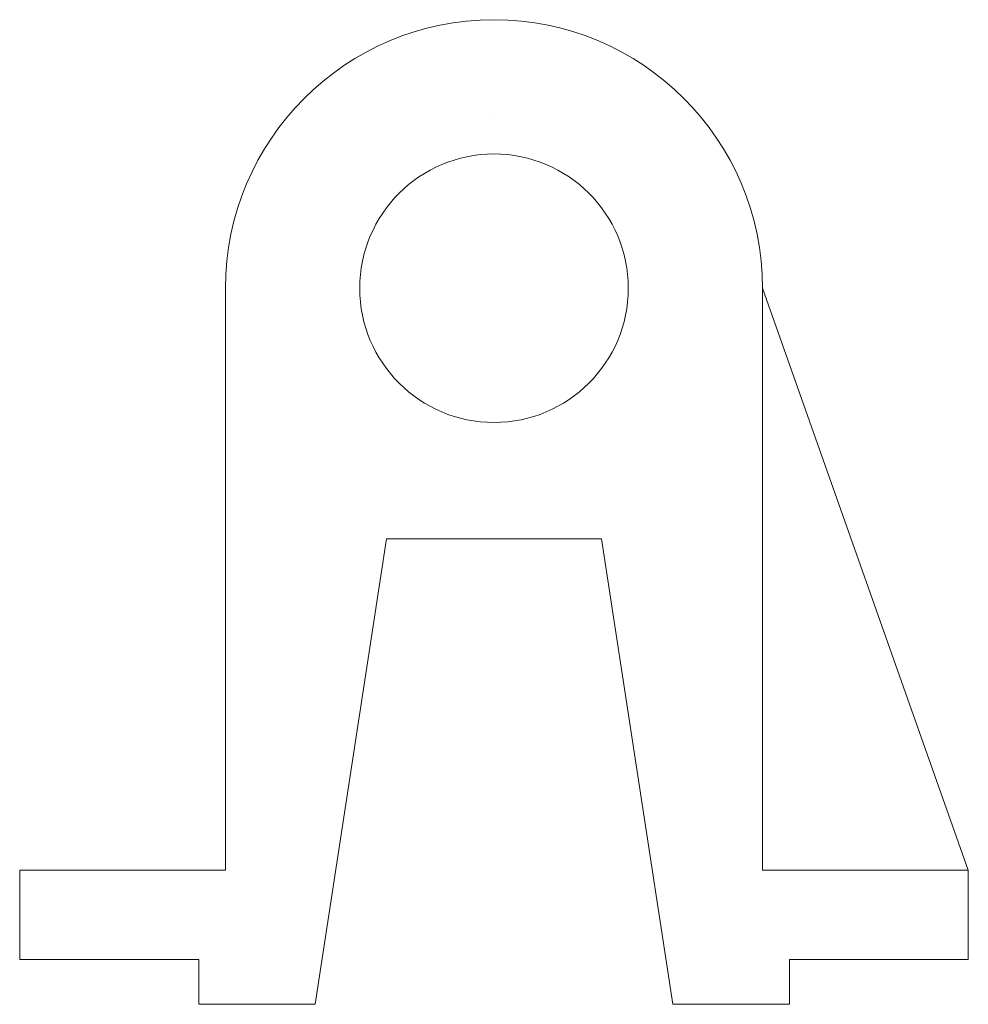
# Model space of a CAD drawing. Units: millimetres. Extents: x 2293 to 2399, y 939 to 1049.
import ezdxf

# ---------------------------------------------------------------- set-up
doc = ezdxf.new("R2010")
doc.units = ezdxf.units.MM
doc.layers.add('M-CONS', color=8, linetype='Continuous', lineweight=13)

msp = doc.modelspace()

# ---------------------------------------------------------------- linework, layer by layer
at = {"layer": 'M-CONS', "extrusion": (0, 1, 0)}
for p, q in [((2345.9, 1038.41, 42), (2345.9, 1038.41, 42)), ((2345.9, 1038.41, 30), (2345.9, 1038.41, 46)), ((2292.9, 954.31, 60), (2304.4, 954.31, 60))]:
    msp.add_line(p, q, dxfattribs=at)
at = {"layer": 'M-CONS'}
for p, q in [((2345.9, 991.31), (2357.9, 991.31)), ((2375.9, 954.31), (2375.9, 954.31, 25)), ((2398.9, 954.31, 60), (2386.9, 954.31, 60))]:
    msp.add_line(p, q, dxfattribs=at)
msp.add_lwpolyline([(2325.9, 939.31), (2312.9, 939.31), (2312.9, 944.31), (2292.9, 944.31), (2292.9, 954.31), (2315.9, 954.31), (2315.9, 1019.31, -1), (2375.9, 1019.31), (2375.9, 954.31), (2398.9, 954.31), (2398.9, 944.31), (2378.9, 944.31), (2378.9, 939.31), (2365.9, 939.31), (2357.9, 991.31), (2333.9, 991.31)], format="xyb", close=True, dxfattribs=at)
at = {"layer": 'M-CONS', "extrusion": (0, 1, 0), "elevation": 1038.41}
msp.add_lwpolyline([(-2345.9, 30), (-2345.9, 30), (-2345.9, 30), (-2345.9, 30)], close=True, dxfattribs=at)
at = {"layer": 'M-CONS', "elevation": 25}
msp.add_lwpolyline([(2375.9, 1019.31), (2375.9, 954.31), (2398.9, 954.31)], close=True, dxfattribs=at)
at = {"layer": 'M-CONS'}
msp.add_circle((2345.9, 1019.31), 15, dxfattribs=at)
at = {"layer": 'M-CONS', "extrusion": (0, 1, 0)}
for centre in [(-2304.4, 48, 954.31), (-2304.4, 12, 954.31), (-2386.9, 48, 954.31), (-2387.4, 12, 954.31)]:
    msp.add_circle(centre, 7.5, dxfattribs=at)

doc.saveas('drawing.dxf')
